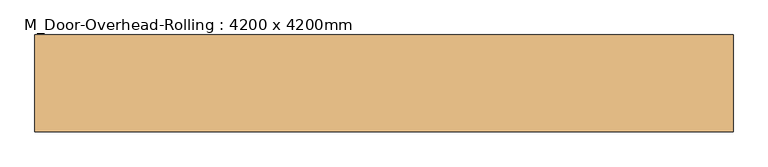
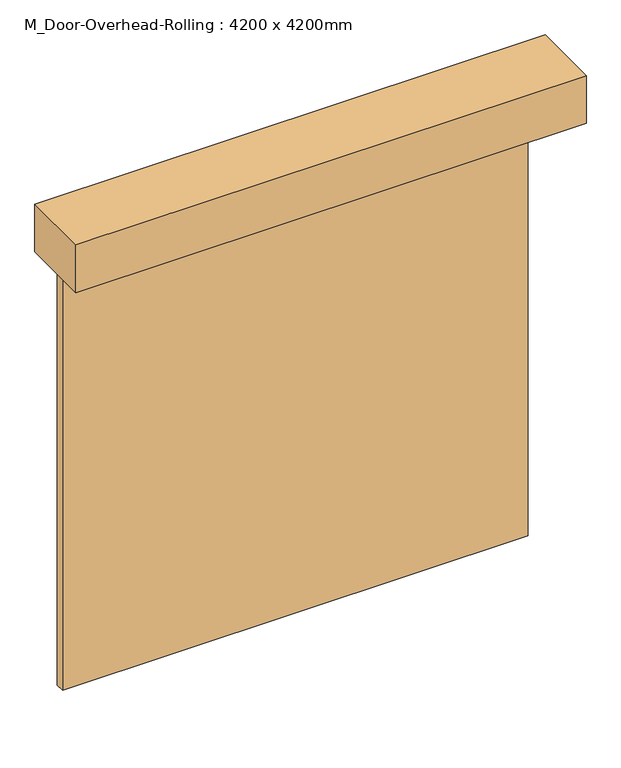
"""IFC4 building model written with IfcOpenShell, lengths in millimetres: door geometry, M_Door-Overhead-Rolling : 4200 x 4200mm."""

from ifc_helpers import new_model, si_unit, frame, origin, origin_with_axes, place, context, project, spatial, polyline, outline, extrude, source, transform, mapped, element, save


def m_door_overhead_rolling_4200_x_4200mm_2c196bb8(model_context):
    return source(origin(), model_context, "Body", "SweptSolid", [
        extrude(outline(polyline([(2100.0, -114.3), (2100.0, -194.3), (-2100.0, -194.3), (-2100.0, -114.3), (2100.0, -114.3)])), origin_with_axes(), (0.0, 0.0, 1.0), 4200.0),
        extrude(outline(polyline([(2303.2, -753.1), (-2303.2, -753.1), (-2303.2, -114.3), (2303.2, -114.3), (2303.2, -753.1)])), frame((0.0, 0.0, 4200.0), z_axis=(0.0, 0.0, 1.0), x_axis=(1.0, 0.0, 0.0)), (0.0, 0.0, 1.0), 457.2),
    ])


if __name__ == "__main__":
    model = new_model("IFC4")
    model_context = context("Model", 3, world=origin())
    ifc_project = project(units=[si_unit("LENGTHUNIT", "METRE", prefix="MILLI")], contexts=[model_context])
    site = spatial("IfcSite", under=ifc_project)
    building = spatial("IfcBuilding", under=site)
    placement = place(None, origin())
    m_door_overhead_rolling_4200_x_4200mm_shape = m_door_overhead_rolling_4200_x_4200mm_2c196bb8(model_context)
    element("IfcDoor", 1, ObjectType="M_Door-Overhead-Rolling : 4200 x 4200mm", at=placement, inside=building, context=model_context, shape_type="MappedRepresentation", body=[
        mapped(m_door_overhead_rolling_4200_x_4200mm_shape, transform((0.0, 0.0, 0.0), x_axis=(1.0, 0.0, 0.0), y_axis=(0.0, 1.0, 0.0), z_axis=(0.0, 0.0, 1.0))),
    ])
    save(model, "model.ifc")

# Revit data of these elements
# Type "M_Door-Overhead-Rolling : 4200 x 4200mm"
#   Type Mark = "40"
#   Construction Type Id = "MDOOR"
#   Assembly Code = "B2030400"
#   Analytic Construction = "Metal"
#   Thickness = 80 mm
#   Rough Width [instance default] = 4200 mm
#   Rough Height [instance default] = 4200 mm
#   Heat Transfer Coefficient (U) = 3.7021 W/(m²·K)
#   Height [instance default] = 4200 mm
#   Width [instance default] = 4200 mm
#   Define Thermal Properties by = 1
#   Function = 1
#   Roller Material = Steel, Paint Finish, Ivory, Matte
#   Roller Box Material = Steel, Paint Finish, Ivory, Matte
#   Visual Light Transmittance = 0
#   Solar Heat Gain Coefficient = 0
#   Wall Closure = (empty or 0)
# Element 1 (IfcDoor, "M_Door-Overhead-Rolling : 4200 x 4200mm")
#   Materials on its faces: "Steel, Paint Finish, Ivory, Matte"
# Materials
#   "Steel, Paint Finish, Ivory, Matte": class "Metal", colour RGB 247 247 239, transparency 0, Description = "Steel, paint finish, ivory, matte", Cost = 0
